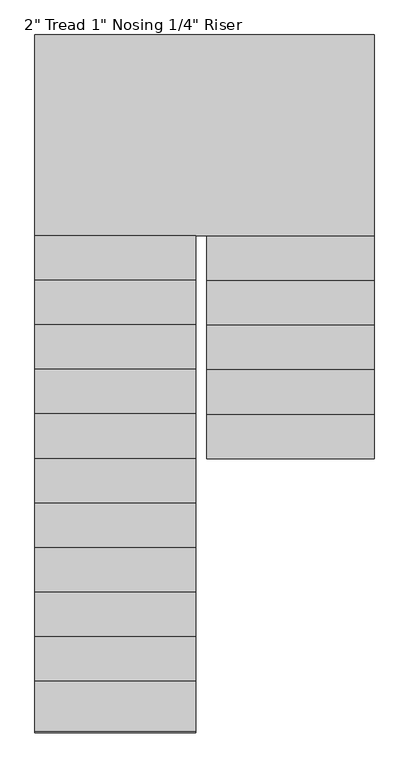
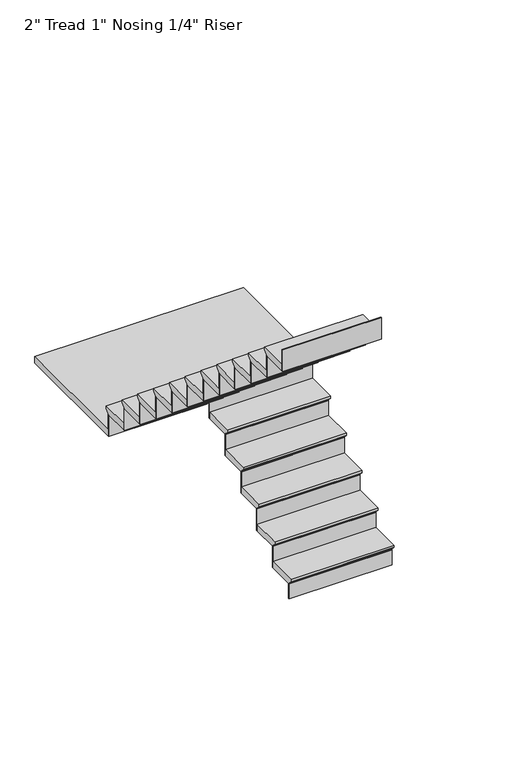
"""IFC4 building model written with IfcOpenShell, lengths in millimetres: stair flight geometry."""

from ifc_helpers import new_model, si_unit, origin, place, context, project, spatial, faceted_brep, source, transform, mapped, element, save


def stair_flight_07a640bc(model_context):
    return source(origin(), model_context, "Body", "Brep", [
        faceted_brep([(-3749.597125, 2714.6319226, 24381.8833333), (-3749.597125, 2714.6319226, 24400.9333333), (-4512.2136682, 2714.6319226, 24400.9333333), (-4512.2136682, 2714.6319226, 24381.8833333), (-3749.597125, 2740.0319226, 24356.4833333), (-4512.2136682, 2740.0319226, 24356.4833333), (-3749.597125, 2943.2319226, 24400.9333333), (-4512.2136682, 2943.2319226, 24400.9333333), (-4512.2136682, 2740.0319226, 24350.1333333), (-4512.2136682, 2943.2319226, 24350.1333333), (-3749.597125, 2943.2319226, 24350.1333333), (-3749.597125, 2740.0319226, 24350.1333333)], [[[0, 1, 2, 3]], [[4, 0, 3, 5]], [[2, 1, 6, 7]], [[8, 9, 10, 11]], [[2, 7, 9, 8, 5, 3]], [[8, 11, 4, 5]], [[6, 1, 0, 4, 11, 10]], [[7, 6, 10, 9]]]),
        faceted_brep([(-3749.597125, 2740.0319226, 24350.1333333), (-3749.597125, 2740.0319226, 24231.6), (-3749.597125, 2746.3819226, 24231.6), (-3749.597125, 2746.3819226, 24350.1333333), (-4512.2136682, 2740.0319226, 24350.1333333), (-4512.2136682, 2746.3819226, 24350.1333333), (-4512.2136682, 2746.3819226, 24231.6), (-4512.2136682, 2740.0319226, 24231.6)], [[[0, 1, 2, 3]], [[4, 5, 6, 7]], [[1, 0, 4, 7]], [[2, 1, 7, 6]], [[3, 2, 6, 5]], [[0, 3, 5, 4]]]),
        faceted_brep([(-3749.597125, 2943.2319226, 24519.4666667), (-3749.597125, 2943.2319226, 24350.1333333), (-3749.597125, 2949.5819226, 24350.1333333), (-3749.597125, 2949.5819226, 24519.4666667), (-4512.2136682, 2943.2319226, 24519.4666667), (-4512.2136682, 2949.5819226, 24519.4666667), (-4512.2136682, 2949.5819226, 24350.1333333), (-4512.2136682, 2943.2319226, 24350.1333333)], [[[0, 1, 2, 3]], [[4, 5, 6, 7]], [[1, 0, 4, 7]], [[2, 1, 7, 6]], [[3, 2, 6, 5]], [[0, 3, 5, 4]]]),
        faceted_brep([(-4512.2136682, 2917.8319226, 24570.2666667), (-3749.597125, 2917.8319226, 24570.2666667), (-3749.597125, 3146.4319226, 24570.2666667), (-4512.2136682, 3146.4319226, 24570.2666667), (-4512.2136682, 2943.2319226, 24519.4666667), (-4512.2136682, 3146.4319226, 24519.4666667), (-3749.597125, 3146.4319226, 24519.4666667), (-3749.597125, 2943.2319226, 24519.4666667), (-4512.2136682, 2943.2319226, 24525.8166667), (-4512.2136682, 2917.8319226, 24551.2166667), (-3749.597125, 2943.2319226, 24525.8166667), (-3749.597125, 2917.8319226, 24551.2166667)], [[[0, 1, 2, 3]], [[4, 5, 6, 7]], [[0, 3, 5, 4, 8, 9]], [[4, 7, 10, 8]], [[2, 1, 11, 10, 7, 6]], [[3, 2, 6, 5]], [[11, 1, 0, 9]], [[10, 11, 9, 8]]]),
        faceted_brep([(-3749.597125, 3146.4319226, 24688.8), (-3749.597125, 3146.4319226, 24519.4666667), (-3749.597125, 3152.7819226, 24519.4666667), (-3749.597125, 3152.7819226, 24688.8), (-4512.2136682, 3146.4319226, 24688.8), (-4512.2136682, 3152.7819226, 24688.8), (-4512.2136682, 3152.7819226, 24519.4666667), (-4512.2136682, 3146.4319226, 24519.4666667)], [[[0, 1, 2, 3]], [[4, 5, 6, 7]], [[1, 0, 4, 7]], [[2, 1, 7, 6]], [[3, 2, 6, 5]], [[0, 3, 5, 4]]]),
        faceted_brep([(-4512.2136682, 3121.0319226, 24739.6), (-3749.597125, 3121.0319226, 24739.6), (-3749.597125, 3349.6319226, 24739.6), (-4512.2136682, 3349.6319226, 24739.6), (-4512.2136682, 3146.4319226, 24688.8), (-4512.2136682, 3349.6319226, 24688.8), (-3749.597125, 3349.6319226, 24688.8), (-3749.597125, 3146.4319226, 24688.8), (-4512.2136682, 3146.4319226, 24695.15), (-4512.2136682, 3121.0319226, 24720.55), (-3749.597125, 3146.4319226, 24695.15), (-3749.597125, 3121.0319226, 24720.55)], [[[0, 1, 2, 3]], [[4, 5, 6, 7]], [[0, 3, 5, 4, 8, 9]], [[4, 7, 10, 8]], [[2, 1, 11, 10, 7, 6]], [[3, 2, 6, 5]], [[11, 1, 0, 9]], [[10, 11, 9, 8]]]),
        faceted_brep([(-3749.597125, 3349.6319226, 24858.1333333), (-3749.597125, 3349.6319226, 24688.8), (-3749.597125, 3355.9819226, 24688.8), (-3749.597125, 3355.9819226, 24858.1333333), (-4512.2136682, 3349.6319226, 24858.1333333), (-4512.2136682, 3355.9819226, 24858.1333333), (-4512.2136682, 3355.9819226, 24688.8), (-4512.2136682, 3349.6319226, 24688.8)], [[[0, 1, 2, 3]], [[4, 5, 6, 7]], [[1, 0, 4, 7]], [[2, 1, 7, 6]], [[3, 2, 6, 5]], [[0, 3, 5, 4]]]),
        faceted_brep([(-4512.2136682, 3324.2319226, 24908.9333333), (-3749.597125, 3324.2319226, 24908.9333333), (-3749.597125, 3552.8319226, 24908.9333333), (-4512.2136682, 3552.8319226, 24908.9333333), (-4512.2136682, 3349.6319226, 24858.1333333), (-4512.2136682, 3552.8319226, 24858.1333333), (-3749.597125, 3552.8319226, 24858.1333333), (-3749.597125, 3349.6319226, 24858.1333333), (-4512.2136682, 3349.6319226, 24864.4833333), (-4512.2136682, 3324.2319226, 24889.8833333), (-3749.597125, 3349.6319226, 24864.4833333), (-3749.597125, 3324.2319226, 24889.8833333)], [[[0, 1, 2, 3]], [[4, 5, 6, 7]], [[0, 3, 5, 4, 8, 9]], [[4, 7, 10, 8]], [[2, 1, 11, 10, 7, 6]], [[3, 2, 6, 5]], [[11, 1, 0, 9]], [[10, 11, 9, 8]]]),
        faceted_brep([(-3749.597125, 3552.8319226, 25027.4666667), (-3749.597125, 3552.8319226, 24858.1333333), (-3749.597125, 3559.1819226, 24858.1333333), (-3749.597125, 3559.1819226, 25027.4666667), (-4512.2136682, 3552.8319226, 25027.4666667), (-4512.2136682, 3559.1819226, 25027.4666667), (-4512.2136682, 3559.1819226, 24858.1333333), (-4512.2136682, 3552.8319226, 24858.1333333)], [[[0, 1, 2, 3]], [[4, 5, 6, 7]], [[1, 0, 4, 7]], [[2, 1, 7, 6]], [[3, 2, 6, 5]], [[0, 3, 5, 4]]]),
        faceted_brep([(-4512.2136682, 3527.4319226, 25078.2666667), (-3749.597125, 3527.4319226, 25078.2666667), (-3749.597125, 3756.0319226, 25078.2666667), (-4512.2136682, 3756.0319226, 25078.2666667), (-4512.2136682, 3552.8319226, 25027.4666667), (-4512.2136682, 3756.0319226, 25027.4666667), (-3749.597125, 3756.0319226, 25027.4666667), (-3749.597125, 3552.8319226, 25027.4666667), (-4512.2136682, 3552.8319226, 25033.8166667), (-4512.2136682, 3527.4319226, 25059.2166667), (-3749.597125, 3552.8319226, 25033.8166667), (-3749.597125, 3527.4319226, 25059.2166667)], [[[0, 1, 2, 3]], [[4, 5, 6, 7]], [[0, 3, 5, 4, 8, 9]], [[4, 7, 10, 8]], [[2, 1, 11, 10, 7, 6]], [[3, 2, 6, 5]], [[11, 1, 0, 9]], [[10, 11, 9, 8]]]),
        faceted_brep([(-3749.597125, 3756.0319226, 25196.8), (-3749.597125, 3756.0319226, 25027.4666667), (-3749.597125, 3762.3819226, 25027.4666667), (-3749.597125, 3762.3819226, 25196.8), (-4512.2136682, 3756.0319226, 25196.8), (-4512.2136682, 3762.3819226, 25196.8), (-4512.2136682, 3762.3819226, 25027.4666667), (-4512.2136682, 3756.0319226, 25027.4666667)], [[[0, 1, 2, 3]], [[4, 5, 6, 7]], [[1, 0, 4, 7]], [[2, 1, 7, 6]], [[3, 2, 6, 5]], [[0, 3, 5, 4]]]),
        faceted_brep([(-4563.0136682, 3705.2319226, 25247.6), (-4563.0136682, 3730.6319226, 25247.6), (-3749.597125, 3730.6319226, 25247.6), (-3749.597125, 4645.0319226, 25247.6), (-5295.0246464, 4645.0319226, 25247.6), (-5295.0246464, 3705.2319226, 25247.6), (-4563.0136682, 3730.6319226, 25196.8), (-4563.0136682, 3705.2319226, 25196.8), (-5295.0246464, 3705.2319226, 25196.8), (-5295.0246464, 4645.0319226, 25196.8), (-3749.597125, 4645.0319226, 25196.8), (-3749.597125, 3756.0319226, 25196.8), (-4512.2136682, 3756.0319226, 25196.8), (-4512.2136682, 3730.6319226, 25196.8), (-4512.2136682, 3730.6319226, 25228.55), (-3749.597125, 3730.6319226, 25228.55), (-4512.2136682, 3756.0319226, 25203.15), (-3749.597125, 3756.0319226, 25203.15)], [[[0, 1, 2, 3, 4, 5]], [[6, 7, 8, 9, 10, 11, 12, 13]], [[1, 0, 7, 6]], [[2, 1, 6, 13, 14, 15]], [[13, 12, 16, 14]], [[12, 11, 17, 16]], [[3, 2, 15, 17, 11, 10]], [[4, 3, 10, 9]], [[5, 4, 9, 8]], [[0, 5, 8, 7]], [[17, 15, 14, 16]]]),
        faceted_brep([(-5295.0246464, 3705.2319226, 25366.1333333), (-5295.0246464, 3705.2319226, 25196.8), (-5295.0246464, 3698.8819226, 25196.8), (-5295.0246464, 3698.8819226, 25366.1333333), (-4563.0136682, 3705.2319226, 25366.1333333), (-4563.0136682, 3698.8819226, 25366.1333333), (-4563.0136682, 3698.8819226, 25196.8), (-4563.0136682, 3705.2319226, 25196.8)], [[[0, 1, 2, 3]], [[4, 5, 6, 7]], [[1, 0, 4, 7]], [[2, 1, 7, 6]], [[3, 2, 6, 5]], [[0, 3, 5, 4]]]),
        faceted_brep([(-4563.0136682, 3730.6319226, 25416.9333333), (-5295.0246464, 3730.6319226, 25416.9333333), (-5295.0246464, 3502.0319226, 25416.9333333), (-4563.0136682, 3502.0319226, 25416.9333333), (-4563.0136682, 3705.2319226, 25366.1333333), (-4563.0136682, 3502.0319226, 25366.1333333), (-5295.0246464, 3502.0319226, 25366.1333333), (-5295.0246464, 3705.2319226, 25366.1333333), (-4563.0136682, 3705.2319226, 25372.4833333), (-4563.0136682, 3730.6319226, 25397.8833333), (-5295.0246464, 3705.2319226, 25372.4833333), (-5295.0246464, 3730.6319226, 25397.8833333)], [[[0, 1, 2, 3]], [[4, 5, 6, 7]], [[0, 3, 5, 4, 8, 9]], [[4, 7, 10, 8]], [[2, 1, 11, 10, 7, 6]], [[3, 2, 6, 5]], [[11, 1, 0, 9]], [[10, 11, 9, 8]]]),
        faceted_brep([(-5295.0246464, 3502.0319226, 25535.4666667), (-5295.0246464, 3502.0319226, 25366.1333333), (-5295.0246464, 3495.6819226, 25366.1333333), (-5295.0246464, 3495.6819226, 25535.4666667), (-4563.0136682, 3502.0319226, 25535.4666667), (-4563.0136682, 3495.6819226, 25535.4666667), (-4563.0136682, 3495.6819226, 25366.1333333), (-4563.0136682, 3502.0319226, 25366.1333333)], [[[0, 1, 2, 3]], [[4, 5, 6, 7]], [[1, 0, 4, 7]], [[2, 1, 7, 6]], [[3, 2, 6, 5]], [[0, 3, 5, 4]]]),
        faceted_brep([(-4563.0136682, 3527.4319226, 25586.2666667), (-5295.0246464, 3527.4319226, 25586.2666667), (-5295.0246464, 3298.8319226, 25586.2666667), (-4563.0136682, 3298.8319226, 25586.2666667), (-4563.0136682, 3502.0319226, 25535.4666667), (-4563.0136682, 3298.8319226, 25535.4666667), (-5295.0246464, 3298.8319226, 25535.4666667), (-5295.0246464, 3502.0319226, 25535.4666667), (-4563.0136682, 3502.0319226, 25541.8166667), (-4563.0136682, 3527.4319226, 25567.2166667), (-5295.0246464, 3502.0319226, 25541.8166667), (-5295.0246464, 3527.4319226, 25567.2166667)], [[[0, 1, 2, 3]], [[4, 5, 6, 7]], [[0, 3, 5, 4, 8, 9]], [[4, 7, 10, 8]], [[2, 1, 11, 10, 7, 6]], [[3, 2, 6, 5]], [[11, 1, 0, 9]], [[10, 11, 9, 8]]]),
        faceted_brep([(-5295.0246464, 3298.8319226, 25704.8), (-5295.0246464, 3298.8319226, 25535.4666667), (-5295.0246464, 3292.4819226, 25535.4666667), (-5295.0246464, 3292.4819226, 25704.8), (-4563.0136682, 3298.8319226, 25704.8), (-4563.0136682, 3292.4819226, 25704.8), (-4563.0136682, 3292.4819226, 25535.4666667), (-4563.0136682, 3298.8319226, 25535.4666667)], [[[0, 1, 2, 3]], [[4, 5, 6, 7]], [[1, 0, 4, 7]], [[2, 1, 7, 6]], [[3, 2, 6, 5]], [[0, 3, 5, 4]]]),
        faceted_brep([(-4563.0136682, 3324.2319226, 25755.6), (-5295.0246464, 3324.2319226, 25755.6), (-5295.0246464, 3095.6319226, 25755.6), (-4563.0136682, 3095.6319226, 25755.6), (-4563.0136682, 3298.8319226, 25704.8), (-4563.0136682, 3095.6319226, 25704.8), (-5295.0246464, 3095.6319226, 25704.8), (-5295.0246464, 3298.8319226, 25704.8), (-4563.0136682, 3298.8319226, 25711.15), (-4563.0136682, 3324.2319226, 25736.55), (-5295.0246464, 3298.8319226, 25711.15), (-5295.0246464, 3324.2319226, 25736.55)], [[[0, 1, 2, 3]], [[4, 5, 6, 7]], [[0, 3, 5, 4, 8, 9]], [[4, 7, 10, 8]], [[2, 1, 11, 10, 7, 6]], [[3, 2, 6, 5]], [[11, 1, 0, 9]], [[10, 11, 9, 8]]]),
        faceted_brep([(-5295.0246464, 3095.6319226, 25874.1333333), (-5295.0246464, 3095.6319226, 25704.8), (-5295.0246464, 3089.2819226, 25704.8), (-5295.0246464, 3089.2819226, 25874.1333333), (-4563.0136682, 3095.6319226, 25874.1333333), (-4563.0136682, 3089.2819226, 25874.1333333), (-4563.0136682, 3089.2819226, 25704.8), (-4563.0136682, 3095.6319226, 25704.8)], [[[0, 1, 2, 3]], [[4, 5, 6, 7]], [[1, 0, 4, 7]], [[2, 1, 7, 6]], [[3, 2, 6, 5]], [[0, 3, 5, 4]]]),
        faceted_brep([(-4563.0136682, 3121.0319226, 25924.9333333), (-5295.0246464, 3121.0319226, 25924.9333333), (-5295.0246464, 2892.4319226, 25924.9333333), (-4563.0136682, 2892.4319226, 25924.9333333), (-4563.0136682, 3095.6319226, 25874.1333333), (-4563.0136682, 2892.4319226, 25874.1333333), (-5295.0246464, 2892.4319226, 25874.1333333), (-5295.0246464, 3095.6319226, 25874.1333333), (-4563.0136682, 3095.6319226, 25880.4833333), (-4563.0136682, 3121.0319226, 25905.8833333), (-5295.0246464, 3095.6319226, 25880.4833333), (-5295.0246464, 3121.0319226, 25905.8833333)], [[[0, 1, 2, 3]], [[4, 5, 6, 7]], [[0, 3, 5, 4, 8, 9]], [[4, 7, 10, 8]], [[2, 1, 11, 10, 7, 6]], [[3, 2, 6, 5]], [[11, 1, 0, 9]], [[10, 11, 9, 8]]]),
        faceted_brep([(-5295.0246464, 2892.4319226, 26043.4666667), (-5295.0246464, 2892.4319226, 25874.1333333), (-5295.0246464, 2886.0819226, 25874.1333333), (-5295.0246464, 2886.0819226, 26043.4666667), (-4563.0136682, 2892.4319226, 26043.4666667), (-4563.0136682, 2886.0819226, 26043.4666667), (-4563.0136682, 2886.0819226, 25874.1333333), (-4563.0136682, 2892.4319226, 25874.1333333)], [[[0, 1, 2, 3]], [[4, 5, 6, 7]], [[1, 0, 4, 7]], [[2, 1, 7, 6]], [[3, 2, 6, 5]], [[0, 3, 5, 4]]]),
        faceted_brep([(-4563.0136682, 2917.8319226, 26094.2666667), (-5295.0246464, 2917.8319226, 26094.2666667), (-5295.0246464, 2689.2319226, 26094.2666667), (-4563.0136682, 2689.2319226, 26094.2666667), (-4563.0136682, 2892.4319226, 26043.4666667), (-4563.0136682, 2689.2319226, 26043.4666667), (-5295.0246464, 2689.2319226, 26043.4666667), (-5295.0246464, 2892.4319226, 26043.4666667), (-4563.0136682, 2892.4319226, 26049.8166667), (-4563.0136682, 2917.8319226, 26075.2166667), (-5295.0246464, 2892.4319226, 26049.8166667), (-5295.0246464, 2917.8319226, 26075.2166667)], [[[0, 1, 2, 3]], [[4, 5, 6, 7]], [[0, 3, 5, 4, 8, 9]], [[4, 7, 10, 8]], [[2, 1, 11, 10, 7, 6]], [[3, 2, 6, 5]], [[11, 1, 0, 9]], [[10, 11, 9, 8]]]),
        faceted_brep([(-5295.0246464, 2689.2319226, 26212.8), (-5295.0246464, 2689.2319226, 26043.4666667), (-5295.0246464, 2682.8819226, 26043.4666667), (-5295.0246464, 2682.8819226, 26212.8), (-4563.0136682, 2689.2319226, 26212.8), (-4563.0136682, 2682.8819226, 26212.8), (-4563.0136682, 2682.8819226, 26043.4666667), (-4563.0136682, 2689.2319226, 26043.4666667)], [[[0, 1, 2, 3]], [[4, 5, 6, 7]], [[1, 0, 4, 7]], [[2, 1, 7, 6]], [[3, 2, 6, 5]], [[0, 3, 5, 4]]]),
        faceted_brep([(-4563.0136682, 2714.6319226, 26263.6), (-5295.0246464, 2714.6319226, 26263.6), (-5295.0246464, 2486.0319226, 26263.6), (-4563.0136682, 2486.0319226, 26263.6), (-4563.0136682, 2689.2319226, 26212.8), (-4563.0136682, 2486.0319226, 26212.8), (-5295.0246464, 2486.0319226, 26212.8), (-5295.0246464, 2689.2319226, 26212.8), (-4563.0136682, 2689.2319226, 26219.15), (-4563.0136682, 2714.6319226, 26244.55), (-5295.0246464, 2689.2319226, 26219.15), (-5295.0246464, 2714.6319226, 26244.55)], [[[0, 1, 2, 3]], [[4, 5, 6, 7]], [[0, 3, 5, 4, 8, 9]], [[4, 7, 10, 8]], [[2, 1, 11, 10, 7, 6]], [[3, 2, 6, 5]], [[11, 1, 0, 9]], [[10, 11, 9, 8]]]),
        faceted_brep([(-5295.0246464, 2486.0319226, 26382.1333333), (-5295.0246464, 2486.0319226, 26212.8), (-5295.0246464, 2479.6819226, 26212.8), (-5295.0246464, 2479.6819226, 26382.1333333), (-4563.0136682, 2486.0319226, 26382.1333333), (-4563.0136682, 2479.6819226, 26382.1333333), (-4563.0136682, 2479.6819226, 26212.8), (-4563.0136682, 2486.0319226, 26212.8)], [[[0, 1, 2, 3]], [[4, 5, 6, 7]], [[1, 0, 4, 7]], [[2, 1, 7, 6]], [[3, 2, 6, 5]], [[0, 3, 5, 4]]]),
        faceted_brep([(-4563.0136682, 2511.4319226, 26432.9333333), (-5295.0246464, 2511.4319226, 26432.9333333), (-5295.0246464, 2282.8319226, 26432.9333333), (-4563.0136682, 2282.8319226, 26432.9333333), (-4563.0136682, 2486.0319226, 26382.1333333), (-4563.0136682, 2282.8319226, 26382.1333333), (-5295.0246464, 2282.8319226, 26382.1333333), (-5295.0246464, 2486.0319226, 26382.1333333), (-4563.0136682, 2486.0319226, 26388.4833333), (-4563.0136682, 2511.4319226, 26413.8833333), (-5295.0246464, 2486.0319226, 26388.4833333), (-5295.0246464, 2511.4319226, 26413.8833333)], [[[0, 1, 2, 3]], [[4, 5, 6, 7]], [[0, 3, 5, 4, 8, 9]], [[4, 7, 10, 8]], [[2, 1, 11, 10, 7, 6]], [[3, 2, 6, 5]], [[11, 1, 0, 9]], [[10, 11, 9, 8]]]),
        faceted_brep([(-5295.0246464, 2282.8319226, 26551.4666667), (-5295.0246464, 2282.8319226, 26382.1333333), (-5295.0246464, 2276.4819226, 26382.1333333), (-5295.0246464, 2276.4819226, 26551.4666667), (-4563.0136682, 2282.8319226, 26551.4666667), (-4563.0136682, 2276.4819226, 26551.4666667), (-4563.0136682, 2276.4819226, 26382.1333333), (-4563.0136682, 2282.8319226, 26382.1333333)], [[[0, 1, 2, 3]], [[4, 5, 6, 7]], [[1, 0, 4, 7]], [[2, 1, 7, 6]], [[3, 2, 6, 5]], [[0, 3, 5, 4]]]),
        faceted_brep([(-4563.0136682, 2308.2319226, 26602.2666667), (-5295.0246464, 2308.2319226, 26602.2666667), (-5295.0246464, 2079.6319226, 26602.2666667), (-4563.0136682, 2079.6319226, 26602.2666667), (-4563.0136682, 2282.8319226, 26551.4666667), (-4563.0136682, 2079.6319226, 26551.4666667), (-5295.0246464, 2079.6319226, 26551.4666667), (-5295.0246464, 2282.8319226, 26551.4666667), (-4563.0136682, 2282.8319226, 26557.8166667), (-4563.0136682, 2308.2319226, 26583.2166667), (-5295.0246464, 2282.8319226, 26557.8166667), (-5295.0246464, 2308.2319226, 26583.2166667)], [[[0, 1, 2, 3]], [[4, 5, 6, 7]], [[0, 3, 5, 4, 8, 9]], [[4, 7, 10, 8]], [[2, 1, 11, 10, 7, 6]], [[3, 2, 6, 5]], [[11, 1, 0, 9]], [[10, 11, 9, 8]]]),
        faceted_brep([(-5295.0246464, 2079.6319226, 26720.8), (-5295.0246464, 2079.6319226, 26551.4666667), (-5295.0246464, 2073.2819226, 26551.4666667), (-5295.0246464, 2073.2819226, 26720.8), (-4563.0136682, 2079.6319226, 26720.8), (-4563.0136682, 2073.2819226, 26720.8), (-4563.0136682, 2073.2819226, 26551.4666667), (-4563.0136682, 2079.6319226, 26551.4666667)], [[[0, 1, 2, 3]], [[4, 5, 6, 7]], [[1, 0, 4, 7]], [[2, 1, 7, 6]], [[3, 2, 6, 5]], [[0, 3, 5, 4]]]),
        faceted_brep([(-4563.0136682, 2105.0319226, 26771.6), (-5295.0246464, 2105.0319226, 26771.6), (-5295.0246464, 1876.4319226, 26771.6), (-4563.0136682, 1876.4319226, 26771.6), (-4563.0136682, 2079.6319226, 26720.8), (-4563.0136682, 1876.4319226, 26720.8), (-5295.0246464, 1876.4319226, 26720.8), (-5295.0246464, 2079.6319226, 26720.8), (-4563.0136682, 2079.6319226, 26727.15), (-4563.0136682, 2105.0319226, 26752.55), (-5295.0246464, 2079.6319226, 26727.15), (-5295.0246464, 2105.0319226, 26752.55)], [[[0, 1, 2, 3]], [[4, 5, 6, 7]], [[0, 3, 5, 4, 8, 9]], [[4, 7, 10, 8]], [[2, 1, 11, 10, 7, 6]], [[3, 2, 6, 5]], [[11, 1, 0, 9]], [[10, 11, 9, 8]]]),
        faceted_brep([(-5295.0246464, 1876.4319226, 26890.1333333), (-5295.0246464, 1876.4319226, 26720.8), (-5295.0246464, 1870.0819226, 26720.8), (-5295.0246464, 1870.0819226, 26890.1333333), (-4563.0136682, 1876.4319226, 26890.1333333), (-4563.0136682, 1870.0819226, 26890.1333333), (-4563.0136682, 1870.0819226, 26720.8), (-4563.0136682, 1876.4319226, 26720.8)], [[[0, 1, 2, 3]], [[4, 5, 6, 7]], [[1, 0, 4, 7]], [[2, 1, 7, 6]], [[3, 2, 6, 5]], [[0, 3, 5, 4]]]),
        faceted_brep([(-4563.0136682, 1901.8319226, 26940.9333333), (-5295.0246464, 1901.8319226, 26940.9333333), (-5295.0246464, 1673.2319226, 26940.9333333), (-4563.0136682, 1673.2319226, 26940.9333333), (-4563.0136682, 1876.4319226, 26890.1333333), (-4563.0136682, 1673.2319226, 26890.1333333), (-5295.0246464, 1673.2319226, 26890.1333333), (-5295.0246464, 1876.4319226, 26890.1333333), (-4563.0136682, 1876.4319226, 26896.4833333), (-4563.0136682, 1901.8319226, 26921.8833333), (-5295.0246464, 1876.4319226, 26896.4833333), (-5295.0246464, 1901.8319226, 26921.8833333)], [[[0, 1, 2, 3]], [[4, 5, 6, 7]], [[0, 3, 5, 4, 8, 9]], [[4, 7, 10, 8]], [[2, 1, 11, 10, 7, 6]], [[3, 2, 6, 5]], [[11, 1, 0, 9]], [[10, 11, 9, 8]]]),
        faceted_brep([(-5295.0246464, 1673.2319226, 27059.4666667), (-5295.0246464, 1673.2319226, 26890.1333333), (-5295.0246464, 1666.8819226, 26890.1333333), (-5295.0246464, 1666.8819226, 27059.4666667), (-4563.0136682, 1673.2319226, 27059.4666667), (-4563.0136682, 1666.8819226, 27059.4666667), (-4563.0136682, 1666.8819226, 26890.1333333), (-4563.0136682, 1673.2319226, 26890.1333333)], [[[0, 1, 2, 3]], [[4, 5, 6, 7]], [[1, 0, 4, 7]], [[2, 1, 7, 6]], [[3, 2, 6, 5]], [[0, 3, 5, 4]]]),
        faceted_brep([(-4563.0136682, 1698.6319226, 27110.2666667), (-5295.0246464, 1698.6319226, 27110.2666667), (-5295.0246464, 1470.0319226, 27110.2666667), (-4563.0136682, 1470.0319226, 27110.2666667), (-4563.0136682, 1673.2319226, 27059.4666667), (-4563.0136682, 1470.0319226, 27059.4666667), (-5295.0246464, 1470.0319226, 27059.4666667), (-5295.0246464, 1673.2319226, 27059.4666667), (-4563.0136682, 1673.2319226, 27065.8166667), (-4563.0136682, 1698.6319226, 27091.2166667), (-5295.0246464, 1673.2319226, 27065.8166667), (-5295.0246464, 1698.6319226, 27091.2166667)], [[[0, 1, 2, 3]], [[4, 5, 6, 7]], [[0, 3, 5, 4, 8, 9]], [[4, 7, 10, 8]], [[2, 1, 11, 10, 7, 6]], [[3, 2, 6, 5]], [[11, 1, 0, 9]], [[10, 11, 9, 8]]]),
        faceted_brep([(-5295.0246464, 1470.0319226, 27228.8), (-5295.0246464, 1470.0319226, 27059.4666667), (-5295.0246464, 1463.6819226, 27059.4666667), (-5295.0246464, 1463.6819226, 27228.8), (-4563.0136682, 1470.0319226, 27228.8), (-4563.0136682, 1463.6819226, 27228.8), (-4563.0136682, 1463.6819226, 27059.4666667), (-4563.0136682, 1470.0319226, 27059.4666667)], [[[0, 1, 2, 3]], [[4, 5, 6, 7]], [[1, 0, 4, 7]], [[2, 1, 7, 6]], [[3, 2, 6, 5]], [[0, 3, 5, 4]]]),
    ])


if __name__ == "__main__":
    model = new_model("IFC4")
    model_context = context("Model", 3, world=origin())
    ifc_project = project(units=[si_unit("LENGTHUNIT", "METRE", prefix="MILLI")], contexts=[model_context])
    site = spatial("IfcSite", under=ifc_project)
    building = spatial("IfcBuilding", under=site)
    placement = place(None, origin())
    stair_flight_shape = stair_flight_07a640bc(model_context)
    element("IfcStairFlight", 1, ObjectType="2\" Tread 1\" Nosing 1/4\" Riser", at=placement, inside=building, context=model_context, shape_type="MappedRepresentation", body=[
        mapped(stair_flight_shape, transform((0.0, 0.0, 0.0), x_axis=(1.0, 0.0, 0.0), y_axis=(0.0, 1.0, 0.0), z_axis=(0.0, 0.0, 1.0))),
    ])
    save(model, "model.ifc")
